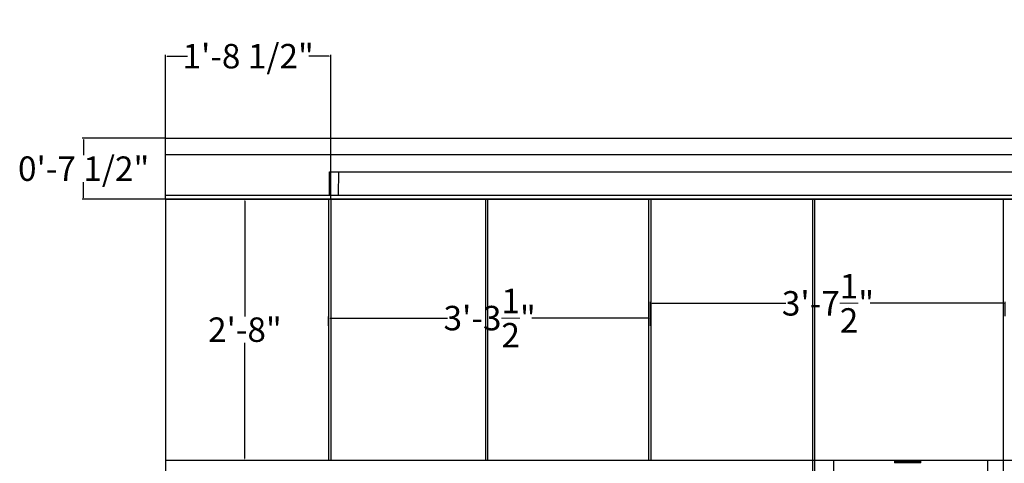
# Model space of a CAD drawing. Units: inches. Extents: x 1686244 to 1686928, y 1936095 to 1936489.
# Tile 4 of 11: x 1686244 to 1686365, y 1936435 to 1936489. Entities that reach past the tile are written whole.
import ezdxf

# ---------------------------------------------------------------- set-up
doc = ezdxf.new("R2010")
doc.units = ezdxf.units.IN
doc.header["$MEASUREMENT"] = 0
for name, color, linetype, lineweight in [('A-ANNO-DIMS', 240, 'Continuous', 18), ('A-ELEV', 7, 'Continuous', 25), ('A-FURN', 40, 'Continuous', 18)]:
    doc.layers.add(name, color=color, linetype=linetype, lineweight=lineweight)
doc.styles.get("Standard").update_dxf_attribs({"font": 'arial.ttf'})
doc.dimstyles.get("Standard").update_dxf_attribs({"dimtxt": 3, "dimasz": 0.18, "dimexe": 0.18, "dimexo": 0.0625, "dimgap": 0.09, "dimtad": 0, "dimtih": 1, "dimtoh": 1, "dimzin": 0, "dimdsep": 46, "dimlunit": 4, "dimtxsty": 'Standard', "dimcen": 0.09, "dimadec": 0, "dimazin": 0, "dimtfac": 1, "dimtofl": 0, "dimtmove": 0, "dimatfit": 3, "dimfxl": 1, "dimtolj": 1, "dimtzin": 0, "dimarcsym": 0})

# ---------------------------------------------------------------- blocks, each defined once
blk = doc.blocks.new('*D1')
at = {"layer": 'A-ANNO-DIMS', "color": 0, "lineweight": -2, "transparency": 16777216}
for p, q in [((1686282.35, 1936451.9), (1686282.35, 1936453.01)), ((1686321.85, 1936451.9), (1686321.85, 1936453.01)), ((1686282.53, 1936452.83), (1686296.93, 1936452.83)), ((1686321.67, 1936452.83), (1686307.27, 1936452.83))]:
    blk.add_line(p, q, dxfattribs=at)
at = {"layer": 'A-ANNO-DIMS', "color": 0, "transparency": 16777216}
for points in [[(1686282.53, 1936452.86), (1686282.53, 1936452.8), (1686282.35, 1936452.83)], [(1686321.67, 1936452.86), (1686321.67, 1936452.8), (1686321.85, 1936452.83)]]:
    blk.add_solid(points, dxfattribs=at)
at = {"layer": 'Defpoints', "color": 0, "transparency": 16777216}
for p in [(1686282.35, 1936451.84), (1686321.85, 1936452.83), (1686321.85, 1936451.84)]:
    blk.add_point(p, dxfattribs=at)
at = {"layer": 'A-ANNO-DIMS', "color": 0, "transparency": 16777216, "insert": (1686302.1, 1936452.83), "char_height": 3, "attachment_point": 5}
blk.add_mtext('\\A1;3\'-3{\\H1x;\\S1/2;}"', dxfattribs=at)
blk = doc.blocks.new('*D5')
at = {"layer": 'A-ANNO-DIMS', "color": 0, "lineweight": -2, "transparency": 16777216}
for p, q in [((1686321.85, 1936453.07), (1686321.85, 1936454.82)), ((1686322.03, 1936454.64), (1686338.43, 1936454.64)), ((1686365.17, 1936454.64), (1686348.77, 1936454.64)), ((1686365.35, 1936453.07), (1686365.35, 1936454.82))]:
    blk.add_line(p, q, dxfattribs=at)
at = {"layer": 'A-ANNO-DIMS', "color": 0, "transparency": 16777216}
for points in [[(1686322.03, 1936454.67), (1686322.03, 1936454.61), (1686321.85, 1936454.64)], [(1686365.17, 1936454.67), (1686365.17, 1936454.61), (1686365.35, 1936454.64)]]:
    blk.add_solid(points, dxfattribs=at)
at = {"layer": 'Defpoints', "color": 0, "transparency": 16777216}
for p in [(1686365.35, 1936454.64), (1686321.85, 1936453.01), (1686365.35, 1936453.01)]:
    blk.add_point(p, dxfattribs=at)
at = {"layer": 'A-ANNO-DIMS', "color": 0, "transparency": 16777216, "insert": (1686343.6, 1936454.64), "char_height": 3, "attachment_point": 5}
blk.add_mtext('\\A1;3\'-7{\\H1x;\\S1/2;}"', dxfattribs=at)
blk = doc.blocks.new('*D6')
at = {"layer": 'A-ANNO-DIMS', "color": 0, "lineweight": -2, "transparency": 16777216}
for p, q in [((1686271.88, 1936467.41), (1686272.26, 1936467.41)), ((1686272.08, 1936467.23), (1686272.08, 1936453.03)), ((1686272.08, 1936435.59), (1686272.08, 1936449.79)), ((1686271.88, 1936435.41), (1686272.26, 1936435.41))]:
    blk.add_line(p, q, dxfattribs=at)
at = {"layer": 'A-ANNO-DIMS', "color": 0, "transparency": 16777216}
for points in [[(1686272.05, 1936467.23), (1686272.11, 1936467.23), (1686272.08, 1936467.41)], [(1686272.05, 1936435.59), (1686272.11, 1936435.59), (1686272.08, 1936435.41)]]:
    blk.add_solid(points, dxfattribs=at)
at = {"layer": 'Defpoints', "color": 0, "transparency": 16777216}
for p in [(1686271.82, 1936467.41), (1686272.08, 1936467.41), (1686271.82, 1936435.41)]:
    blk.add_point(p, dxfattribs=at)
at = {"layer": 'A-ANNO-DIMS', "color": 0, "transparency": 16777216, "insert": (1686272.08, 1936451.41), "char_height": 3, "attachment_point": 5}
blk.add_mtext('\\A1;2\'-8"', dxfattribs=at)
blk = doc.blocks.new('*D92')
at = {"layer": 'A-ANNO-DIMS', "color": 0, "lineweight": -2, "transparency": 16777216}
for p, q in [((1686262.35, 1936467.47), (1686262.35, 1936485.14)), ((1686262.53, 1936484.96), (1686265.05, 1936484.96)), ((1686282.42, 1936484.96), (1686279.91, 1936484.96)), ((1686282.6, 1936467.47), (1686282.6, 1936485.14))]:
    blk.add_line(p, q, dxfattribs=at)
at = {"layer": 'A-ANNO-DIMS', "color": 0, "transparency": 16777216}
for points in [[(1686262.53, 1936484.99), (1686262.53, 1936484.93), (1686262.35, 1936484.96)], [(1686282.42, 1936484.99), (1686282.42, 1936484.93), (1686282.6, 1936484.96)]]:
    blk.add_solid(points, dxfattribs=at)
at = {"layer": 'Defpoints', "color": 0, "transparency": 16777216}
for p in [(1686282.6, 1936484.96), (1686262.35, 1936467.41), (1686282.6, 1936467.41)]:
    blk.add_point(p, dxfattribs=at)
at = {"layer": 'A-ANNO-DIMS', "color": 0, "transparency": 16777216, "insert": (1686272.48, 1936484.96), "char_height": 3, "attachment_point": 5}
blk.add_mtext('\\A1;1\'-8 1/2"', dxfattribs=at)
blk = doc.blocks.new('*D95')
at = {"layer": 'A-ANNO-DIMS', "color": 0, "lineweight": -2, "transparency": 16777216}
for p, q in [((1686262.29, 1936474.91), (1686252.12, 1936474.91)), ((1686252.3, 1936474.73), (1686252.3, 1936472.8)), ((1686252.3, 1936467.59), (1686252.3, 1936469.52)), ((1686262.29, 1936467.41), (1686252.12, 1936467.41))]:
    blk.add_line(p, q, dxfattribs=at)
at = {"layer": 'A-ANNO-DIMS', "color": 0, "transparency": 16777216}
for points in [[(1686252.27, 1936474.73), (1686252.33, 1936474.73), (1686252.3, 1936474.91)], [(1686252.27, 1936467.59), (1686252.33, 1936467.59), (1686252.3, 1936467.41)]]:
    blk.add_solid(points, dxfattribs=at)
at = {"layer": 'Defpoints', "color": 0, "transparency": 16777216}
for p in [(1686262.35, 1936474.91), (1686252.3, 1936467.41), (1686262.35, 1936467.41)]:
    blk.add_point(p, dxfattribs=at)
at = {"layer": 'A-ANNO-DIMS', "color": 0, "transparency": 16777216, "insert": (1686252.3, 1936471.16), "char_height": 3, "attachment_point": 5}
blk.add_mtext('\\A1;0\'-7 1/2"', dxfattribs=at)

msp = doc.modelspace()

# ---------------------------------------------------------------- linework, layer by layer
at = {"layer": 'A-ELEV'}
for p, q in [((1686262.353, 1936467.412), (1686262.353, 1936474.912)), ((1686262.353, 1936474.912), (1686459.353, 1936474.912)), ((1686262.353, 1936472.912), (1686459.353, 1936472.912)), ((1686282.448, 1936470.78), (1686449.069, 1936470.78)), ((1686282.448, 1936467.912), (1686282.448, 1936470.78)), ((1686283.561, 1936467.912), (1686283.606, 1936470.78)), ((1686262.353, 1936467.912), (1686459.353, 1936467.912)), ((1686262.353, 1936467.412), (1686459.353, 1936467.412)), ((1686282.353, 1936467.412), (1686282.353, 1936435.412)), ((1686282.603, 1936467.412), (1686282.603, 1936435.412)), ((1686301.603, 1936467.412), (1686301.603, 1936435.412)), ((1686301.853, 1936467.412), (1686301.853, 1936435.412)), ((1686321.603, 1936467.412), (1686321.603, 1936435.412)), ((1686321.853, 1936467.412), (1686321.853, 1936435.412)), ((1686341.693, 1936467.412), (1686341.693, 1936357.412)), ((1686341.943, 1936467.412), (1686341.943, 1936357.412)), ((1686365.103, 1936467.412), (1686365.103, 1936357.412)), ((1686262.353, 1936435.412), (1686459.353, 1936435.412)), ((1686344.26, 1936435.412), (1686363.15, 1936435.412)), ((1686344.26, 1936435.412), (1686344.495, 1936357.412)), ((1686363.15, 1936435.412), (1686363.15, 1936358.215))]:
    msp.add_line(p, q, dxfattribs=at)
msp.add_lwpolyline([(1686459.353, 1936357.412), (1686459.353, 1936467.412), (1686262.353, 1936467.412), (1686262.353, 1936357.412)], close=True, dxfattribs=at)
at = {"layer": 'A-FURN'}
for points in [[(1686351.772, 1936435.259), (1686355.006, 1936435.261), (1686355.006, 1936435.083), (1686351.772, 1936435.082)], [(1686351.792, 1936435.239), (1686354.986, 1936435.241), (1686354.986, 1936435.103), (1686351.792, 1936435.102)]]:
    msp.add_lwpolyline(points, close=True, dxfattribs=at)

# ---------------------------------------------------------------- dimensions: what is measured, and where the dimension line sits
at = {"layer": 'A-ANNO-DIMS'}
for base, p1, p2, override, picture, middle in [((1686282.6033, 1936484.9619), (1686262.3528, 1936467.4119), (1686282.6033, 1936467.4119), {"dimdec": 1, "dimlfac": 1, "dimrnd": 0, "dimzin": 1, "dimdsep": 46, "dimlunit": 4, "dimfrac": 2}, '*D92', (1686272.4781, 1936484.9619)), ((1686365.353, 1936454.64), (1686321.853, 1936453.01), (1686365.353, 1936453.01), {"dimclrd": 0, "dimclre": 0, "dimclrt": 0}, '*D5', (1686343.603, 1936454.64)), ((1686321.853, 1936452.83), (1686282.353, 1936451.84), (1686321.853, 1936451.84), {"dimclrd": 0, "dimclre": 0, "dimclrt": 0}, '*D1', (1686302.103, 1936452.83))]:
    dim = msp.add_linear_dim(base=base, p1=p1, p2=p2, dimstyle='Standard', override=override, dxfattribs=at)
    dim.commit()
    dim.dimension.update_dxf_attribs({"geometry": picture, "text_midpoint": middle})
for base, p1, p2, override, picture, middle in [((1686252.303, 1936467.412), (1686262.353, 1936474.912), (1686262.353, 1936467.412), {"dimdec": 1, "dimlfac": 1, "dimrnd": 0, "dimzin": 1, "dimdsep": 46, "dimlunit": 4, "dimfrac": 2}, '*D95', (1686252.303, 1936471.162)), ((1686272.081, 1936467.412), (1686271.822, 1936435.412), (1686271.822, 1936467.412), {"dimclrd": 0, "dimclre": 0, "dimclrt": 0}, '*D6', (1686272.081, 1936451.412))]:
    dim = msp.add_linear_dim(base=base, p1=p1, p2=p2, angle=90, dimstyle='Standard', override=override, dxfattribs=at)
    dim.commit()
    dim.dimension.update_dxf_attribs({"geometry": picture, "text_midpoint": middle})

doc.saveas('drawing.dxf')
